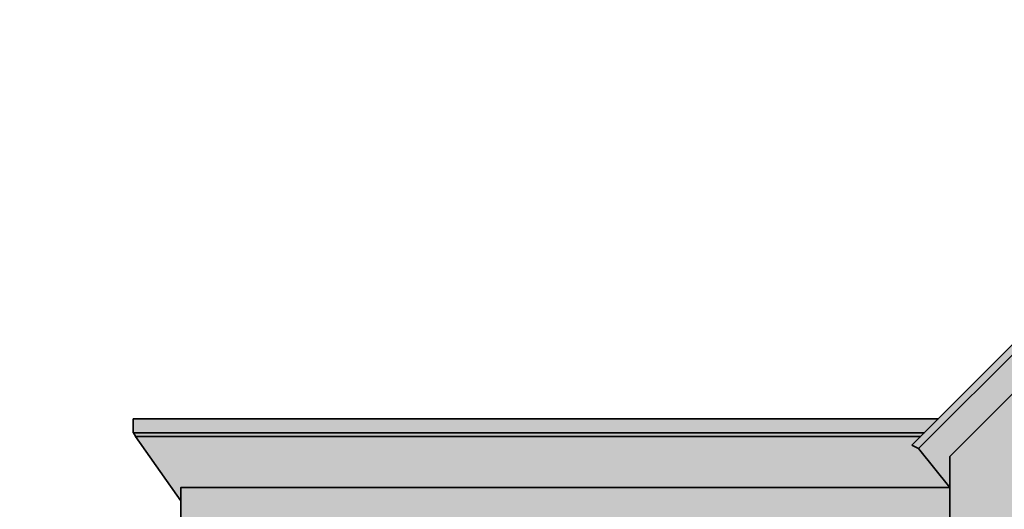
# Model space of a CAD drawing. Units: feet. Extents: x 2613 to 3913, y 950 to 1393.
# Tile 4 of 6: x 2613 to 2948, y 1226 to 1393. Entities that reach past the tile are written whole.
import ezdxf

# ---------------------------------------------------------------- set-up
doc = ezdxf.new("R2010")
doc.units = ezdxf.units.FT
for name, color, linetype, lineweight in [('A-ELEV', 7, 'Continuous', 35), ('A-ELEV-PATT', 9, 'Continuous', 13), ('A-ROOF', 1, 'Continuous', 35)]:
    doc.layers.add(name, color=color, linetype=linetype, lineweight=lineweight)

msp = doc.modelspace()

# ---------------------------------------------------------------- hatches: boundary and pattern name
at = {"layer": 'A-ELEV-PATT'}
h = msp.add_hatch(color=256, dxfattribs=at)
h.dxf.hatch_style = 1
h.paths.add_polyline_path([(3108.91, 1328.81), (3061.44, 1376.28), (2929.45, 1244.29), (2929.45, 1223.38), (2942.09, 1223.38), (2942.09, 1215.5), (2929.45, 1215.5), (2929.45, 1084.12), (3108.91, 1084.12), (3108.91, 1199.69), (3106.87, 1199.69), (3106.87, 1128.72), (3017.91, 1128.72), (3017.91, 1199.69), (3008.08, 1199.69), (3008.08, 1180.01), (3007.65, 1180.01), (3007.65, 1199.69), (3004.75, 1199.69), (3004.75, 1206.47), (3108.91, 1206.47)])
h.paths.add_polyline_path([(3061.44, 1376.28), (3193.8, 1243.92), (3193.8, 1233.84), (3204.34, 1246.9), (3061.54, 1389.71), (2918.82, 1247), (2929.45, 1233.69), (2929.45, 1244.29)])
h.paths.add_polyline_path([(3061.54, 1389.71), (3204.34, 1246.9), (3206.69, 1248.02), (3061.63, 1393.09), (2916.59, 1248.06), (2918.82, 1247)])
h.paths.add_polyline_path([(2925.65, 1257.12), (2667.59, 1257.12), (2651.33, 1257.12), (2651.33, 1252.28), (2920.82, 1252.28)])
h.paths.add_polyline_path([(2920.82, 1252.28), (2651.33, 1252.28, -0.144454), (2652.15, 1251.12), (2667.59, 1251.12), (2919.65, 1251.12)])
h.paths.add_polyline_path([(2918.82, 1247), (2916.59, 1248.06), (2919.65, 1251.12), (2667.59, 1251.12), (2652.15, 1251.12), (2667.59, 1229.14), (2667.59, 1233.69), (2929.45, 1233.69)])
h.paths.add_polyline_path([(2710.6, 1223.38), (2929.45, 1223.38), (2929.45, 1233.69), (2667.59, 1233.69), (2667.59, 1229.14), (2667.59, 1201.16), (2720.67, 1201.16), (2710.6, 1215.5)])
h.paths.add_polyline_path([(2942.09, 1223.38), (2710.6, 1223.38), (2710.6, 1215.5), (2921.48, 1215.5), (2942.09, 1215.5)])
h.paths.add_polyline_path([(2929.45, 1215.5), (2921.48, 1215.5), (2710.6, 1215.5), (2733.47, 1182.94), (2733.47, 1195.74), (2741.22, 1195.74), (2929.45, 1195.74)])
h.paths.add_polyline_path([(2721, 1200.68), (2661.89, 1200.68), (2661.89, 1195.74), (2724.47, 1195.74)])
h.paths.add_polyline_path([(2733.47, 1182.94), (2727.27, 1191.76), (2727.27, 1133.88), (2731.7, 1133.88), (2731.7, 1169.74), (2731.61, 1169.74), (2731.61, 1170.13), (2733.47, 1170.13)])
h.paths.add_polyline_path([(2929.45, 1183.04), (2741.22, 1183.04), (2741.22, 1170.13), (2743.07, 1170.13), (2743.07, 1169.74), (2743.07, 1112.32), (2759.57, 1112.32), (2759.57, 1167.82), (2763.7, 1167.82), (2763.7, 1112.32), (2781.75, 1112.32), (2781.75, 1167.82), (2785.87, 1167.82), (2785.87, 1112.32), (2803.92, 1112.32), (2803.92, 1167.82), (2808.05, 1167.82), (2808.05, 1112.32), (2826.09, 1112.32), (2826.09, 1167.82), (2830.22, 1167.82), (2830.22, 1112.32), (2875.17, 1112.32), (2875.17, 1171.49), (2929.45, 1171.49)])
h.paths.add_polyline_path([(2731.7, 1133.88), (2661.89, 1133.88), (2661.89, 1084.12), (2730.99, 1084.12), (2730.99, 1112.32), (2731.7, 1112.32)])
h.paths.add_polyline_path([(2929.45, 1112.32), (2730.99, 1112.32), (2730.99, 1084.12), (2929.45, 1084.12)])
h.paths.add_polyline_path([(2929.45, 1084.12), (2730.99, 1084.12), (2661.89, 1084.12), (2612.72, 1084.12), (2612.72, 1082.68), (2929.45, 1082.68)])
h.paths.add_polyline_path([(2929.45, 1082.68), (2612.72, 1082.68), (2639.32, 1062.44), (2733.47, 1062.44), (2733.47, 1063.35), (2639.62, 1063.35), (2615.43, 1081.77), (2723.91, 1081.77), (2739.71, 1069.74), (2741.22, 1069.74), (2725.42, 1081.77), (2929.45, 1081.77)])
h.paths.add_polyline_path([(2671.42, 1081.77), (2668.07, 1081.77), (2692.27, 1063.35), (2695.62, 1063.35)], flags=17)
h.paths.add_polyline_path([(2741.22, 1069.74), (2741.22, 1068.59), (2748.11, 1063.35), (2741.22, 1063.35), (2741.22, 1062.44), (2750.82, 1062.44)], flags=17)
h.paths.add_polyline_path([(2929.45, 1081.77), (2725.42, 1081.77), (2750.82, 1062.44), (2741.22, 1062.44), (2741.22, 1047.95), (2743.07, 1047.95), (2743.07, 1047.56), (2743.07, 967.97), (2875.17, 967.97), (2875.17, 1066.37), (2929.45, 1066.37)])
h.paths.add_polyline_path([(2778.55, 1066.37), (2806.94, 1066.37), (2806.94, 982.04), (2778.55, 982.04)], flags=16)
h.paths.add_polyline_path([(2778.55, 1064.05), (2806.94, 1064.05), (2806.94, 1063.39), (2778.55, 1063.39)], flags=16)
h.paths.add_polyline_path([(2778.55, 1061.07), (2806.94, 1061.07), (2806.94, 1060.41), (2778.55, 1060.41)], flags=0)
h.paths.add_polyline_path([(2778.55, 1058.09), (2806.94, 1058.09), (2806.94, 1057.43), (2778.55, 1057.43)], flags=0)
h.paths.add_polyline_path([(2778.55, 1055.11), (2806.94, 1055.11), (2806.94, 1054.45), (2778.55, 1054.45)], flags=0)
h.paths.add_polyline_path([(2778.55, 1052.13), (2806.94, 1052.13), (2806.94, 1051.47), (2778.55, 1051.47)], flags=0)
h.paths.add_polyline_path([(2778.55, 1049.15), (2806.94, 1049.15), (2806.94, 1048.49), (2778.55, 1048.49)], flags=0)
h.paths.add_polyline_path([(2778.55, 1046.18), (2806.94, 1046.18), (2806.94, 1045.51), (2778.55, 1045.51)], flags=0)
h.paths.add_polyline_path([(2778.55, 1043.2), (2806.94, 1043.2), (2806.94, 1042.53), (2778.55, 1042.53)], flags=0)
h.paths.add_polyline_path([(2778.55, 1040.22), (2806.94, 1040.22), (2806.94, 1039.56), (2778.55, 1039.56)], flags=0)
h.paths.add_polyline_path([(2778.55, 1037.24), (2806.94, 1037.24), (2806.94, 1036.58), (2778.55, 1036.58)], flags=0)
h.paths.add_polyline_path([(2778.55, 1034.26), (2806.94, 1034.26), (2806.94, 1033.6), (2778.55, 1033.6)], flags=0)
h.paths.add_polyline_path([(2778.55, 1031.28), (2806.94, 1031.28), (2806.94, 1030.62), (2778.55, 1030.62)], flags=0)
h.paths.add_polyline_path([(2778.55, 1028.3), (2806.94, 1028.3), (2806.94, 1027.64), (2778.55, 1027.64)], flags=0)
h.paths.add_polyline_path([(2778.55, 1025.32), (2806.94, 1025.32), (2806.94, 1024.66), (2778.55, 1024.66)], flags=0)
h.paths.add_polyline_path([(2778.55, 1022.34), (2806.94, 1022.34), (2806.94, 1021.68), (2778.55, 1021.68)], flags=0)
h.paths.add_polyline_path([(2778.55, 1019.36), (2806.94, 1019.36), (2806.94, 1018.7), (2778.55, 1018.7)], flags=0)
h.paths.add_polyline_path([(2778.55, 1016.71), (2806.94, 1016.71), (2806.94, 1016.05), (2778.55, 1016.05)], flags=0)
h.paths.add_polyline_path([(2824.02, 1066.37), (2852.41, 1066.37), (2852.41, 982.04), (2824.02, 982.04)], flags=16)
h.paths.add_polyline_path([(2778.55, 1014.07), (2806.94, 1014.07), (2806.94, 1013.4), (2778.55, 1013.4)], flags=0)
h.paths.add_polyline_path([(2824.02, 1064.05), (2852.41, 1064.05), (2852.41, 1063.39), (2824.02, 1063.39)], flags=16)
h.paths.add_polyline_path([(2824.02, 1061.07), (2852.41, 1061.07), (2852.41, 1060.41), (2824.02, 1060.41)], flags=0)
h.paths.add_polyline_path([(2824.02, 1058.09), (2852.41, 1058.09), (2852.41, 1057.43), (2824.02, 1057.43)], flags=0)
h.paths.add_polyline_path([(2824.02, 1055.11), (2852.41, 1055.11), (2852.41, 1054.45), (2824.02, 1054.45)], flags=16)
h.paths.add_polyline_path([(2824.02, 1052.13), (2852.41, 1052.13), (2852.41, 1051.47), (2824.02, 1051.47)], flags=0)
h.paths.add_polyline_path([(2778.55, 1011.09), (2806.94, 1011.09), (2806.94, 1010.43), (2778.55, 1010.43)], flags=0)
h.paths.add_polyline_path([(2824.02, 1049.15), (2852.41, 1049.15), (2852.41, 1048.49), (2824.02, 1048.49)], flags=0)
h.paths.add_polyline_path([(2824.02, 1046.18), (2852.41, 1046.18), (2852.41, 1045.51), (2824.02, 1045.51)], flags=0)
h.paths.add_polyline_path([(2824.02, 1043.2), (2852.41, 1043.2), (2852.41, 1042.53), (2824.02, 1042.53)], flags=0)
h.paths.add_polyline_path([(2778.55, 1008.11), (2806.94, 1008.11), (2806.94, 1007.45), (2778.55, 1007.45)], flags=0)
h.paths.add_polyline_path([(2824.02, 1040.22), (2852.41, 1040.22), (2852.41, 1039.56), (2824.02, 1039.56)], flags=0)
h.paths.add_polyline_path([(2824.02, 1037.24), (2852.41, 1037.24), (2852.41, 1036.58), (2824.02, 1036.58)], flags=0)
h.paths.add_polyline_path([(2778.55, 1005.13), (2806.94, 1005.13), (2806.94, 1004.47), (2778.55, 1004.47)], flags=0)
h.paths.add_polyline_path([(2824.02, 1034.26), (2852.41, 1034.26), (2852.41, 1033.6), (2824.02, 1033.6)], flags=0)
h.paths.add_polyline_path([(2824.02, 1031.28), (2852.41, 1031.28), (2852.41, 1030.62), (2824.02, 1030.62)], flags=0)
h.paths.add_polyline_path([(2778.55, 1002.15), (2806.94, 1002.15), (2806.94, 1001.49), (2778.55, 1001.49)], flags=0)
h.paths.add_polyline_path([(2824.02, 1028.3), (2852.41, 1028.3), (2852.41, 1027.64), (2824.02, 1027.64)], flags=0)
h.paths.add_polyline_path([(2778.55, 999.17), (2806.94, 999.17), (2806.94, 998.51), (2778.55, 998.51)], flags=0)
h.paths.add_polyline_path([(2824.02, 1025.32), (2852.41, 1025.32), (2852.41, 1024.66), (2824.02, 1024.66)], flags=0)
h.paths.add_polyline_path([(2824.02, 1022.34), (2852.41, 1022.34), (2852.41, 1021.68), (2824.02, 1021.68)], flags=0)
h.paths.add_polyline_path([(2778.55, 996.19), (2806.94, 996.19), (2806.94, 995.53), (2778.55, 995.53)], flags=0)
h.paths.add_polyline_path([(2824.02, 1019.36), (2852.41, 1019.36), (2852.41, 1018.7), (2824.02, 1018.7)], flags=0)
h.paths.add_polyline_path([(2778.55, 993.21), (2806.94, 993.21), (2806.94, 992.55), (2778.55, 992.55)], flags=0)
h.paths.add_polyline_path([(2824.02, 1016.38), (2852.41, 1016.38), (2852.41, 1015.72), (2824.02, 1015.72)], flags=0)
h.paths.add_polyline_path([(2824.02, 1013.4), (2852.41, 1013.4), (2852.41, 1012.74), (2824.02, 1012.74)], flags=0)
h.paths.add_polyline_path([(2778.55, 990.23), (2806.94, 990.23), (2806.94, 989.57), (2778.55, 989.57)], flags=0)
h.paths.add_polyline_path([(2824.02, 1010.43), (2852.41, 1010.43), (2852.41, 1009.76), (2824.02, 1009.76)], flags=0)
h.paths.add_polyline_path([(2778.55, 987.25), (2806.94, 987.25), (2806.94, 986.59), (2778.55, 986.59)], flags=0)
h.paths.add_polyline_path([(2824.02, 1007.45), (2852.41, 1007.45), (2852.41, 1006.78), (2824.02, 1006.78)], flags=0)
h.paths.add_polyline_path([(2778.55, 984.27), (2806.94, 984.27), (2806.94, 983.61), (2778.55, 983.61)], flags=0)
h.paths.add_polyline_path([(2824.02, 1004.47), (2852.41, 1004.47), (2852.41, 1003.81), (2824.02, 1003.81)], flags=0)
h.paths.add_polyline_path([(2824.02, 1001.49), (2852.41, 1001.49), (2852.41, 1000.83), (2824.02, 1000.83)], flags=0)
h.paths.add_polyline_path([(2824.02, 998.51), (2852.41, 998.51), (2852.41, 997.85), (2824.02, 997.85)], flags=0)
h.paths.add_polyline_path([(2824.02, 995.53), (2852.41, 995.53), (2852.41, 994.87), (2824.02, 994.87)], flags=0)
h.paths.add_polyline_path([(2824.02, 992.55), (2852.41, 992.55), (2852.41, 991.89), (2824.02, 991.89)], flags=0)
h.paths.add_polyline_path([(2824.02, 989.57), (2852.41, 989.57), (2852.41, 988.91), (2824.02, 988.91)], flags=0)
h.paths.add_polyline_path([(2824.02, 986.59), (2852.41, 986.59), (2852.41, 985.93), (2824.02, 985.93)], flags=0)
h.paths.add_polyline_path([(2824.02, 983.61), (2852.41, 983.61), (2852.41, 982.95), (2824.02, 982.95)], flags=0)
h.paths.add_polyline_path([(2731.7, 1047.56), (2731.61, 1047.56), (2731.61, 1047.95), (2733.47, 1047.95), (2733.47, 1062.44), (2727.27, 1062.44), (2727.27, 1000.58), (2667.59, 1000.58), (2667.59, 1062.44), (2664.87, 1062.44), (2664.87, 965.01), (2730.76, 964.93), (2730.76, 967.97), (2731.7, 967.97)])
h.paths.add_polyline_path([(2728.06, 961.9), (2730.76, 961.9), (2730.76, 964.93), (2663.94, 964.93), (2663.94, 949.74), (2725.36, 949.74), (2725.36, 955.82), (2728.06, 955.82)])
h.paths.add_polyline_path([(2929.45, 967.97), (2730.76, 967.97), (2730.76, 961.9), (2929.45, 961.9)])
h.paths.add_polyline_path([(2929.45, 961.9), (2730.76, 961.9), (2728.06, 961.9), (2728.06, 955.82), (2929.45, 955.82)])
h.paths.add_polyline_path([(2929.45, 955.82), (2728.06, 955.82), (2725.36, 955.82), (2725.36, 949.74), (2929.45, 949.74)])
h.paths.add_polyline_path([(2741.22, 1069.74), (2733.47, 1069.74), (2733.47, 1047.95), (2741.22, 1047.95)], flags=17)
h.paths.add_polyline_path([(2741.22, 1195.74), (2733.47, 1195.74), (2733.47, 1182.94), (2733.47, 1170.13), (2741.22, 1170.13), (2741.22, 1183.04)])
h.paths.add_polyline_path([(3193.8, 1084.12), (2929.45, 1084.12), (2929.45, 1082.68), (2929.45, 1081.77), (2929.45, 1066.37), (2929.45, 949.74), (3193.8, 949.74)])
h.paths.add_polyline_path([(2937.79, 1075.78), (3185.46, 1075.78), (3185.46, 958.09), (2937.79, 958.09)], flags=16)
h.paths.add_polyline_path([(3011.76, 1075.78), (3104.46, 1075.78), (3104.46, 993.6), (3011.76, 993.6)], flags=0)
h.paths.add_polyline_path([(3015.24, 1075.78), (3016.57, 1075.78), (3016.57, 1060.85), (3043.1, 1060.85), (3043.1, 1075.78), (3045.77, 1075.78), (3045.77, 997.08), (3070.45, 997.08), (3070.45, 1075.78), (3073.12, 1075.78), (3073.12, 1060.85), (3099.64, 1060.85), (3099.64, 1075.78), (3100.98, 1075.78), (3100.98, 997.08), (3099.64, 997.08), (3015.24, 997.08)], flags=0)

# ---------------------------------------------------------------- linework, layer by layer
at = {"layer": 'A-ELEV'}
for p, q in [((2667.59, 1229.14), (2652.15, 1251.12)), ((2667.59, 1229.14), (2652.15, 1251.12)), ((2929.45, 1233.69), (2918.82, 1247)), ((2929.45, 1233.69), (2918.82, 1247))]:
    msp.add_line(p, q, dxfattribs=at)
for points in [[(2929.45, 1244.29), (2929.45, 1223.38)], [(2929.45, 1244.29), (2929.45, 1223.38)], [(2929.45, 1233.69), (2667.59, 1233.69), (2667.59, 1229.14), (2667.59, 1201.16)], [(2929.45, 1233.69), (2667.59, 1233.69), (2667.59, 1229.14), (2667.59, 1201.16)]]:
    msp.add_lwpolyline(points, dxfattribs=at)
at = {"layer": 'A-ROOF'}
for p, q in [((3061.54, 1389.71), (2918.82, 1247)), ((3061.54, 1389.71), (2918.82, 1247)), ((2929.45, 1244.29), (3061.44, 1376.28)), ((2929.45, 1244.29), (3061.44, 1376.28)), ((2667.59, 1257.12), (2651.33, 1257.12)), ((2651.33, 1252.28), (2651.33, 1257.12)), ((2667.59, 1257.12), (2651.33, 1257.12)), ((2651.33, 1252.28), (2651.33, 1257.12)), ((2925.65, 1257.12), (2667.59, 1257.12)), ((2925.65, 1257.12), (2667.59, 1257.12)), ((2920.82, 1252.28), (2651.33, 1252.28)), ((2920.82, 1252.28), (2651.33, 1252.28)), ((2667.59, 1251.12), (2652.15, 1251.12)), ((2667.59, 1251.12), (2652.15, 1251.12)), ((2667.59, 1251.12), (2919.65, 1251.12)), ((2667.59, 1251.12), (2919.65, 1251.12)), ((2918.82, 1247), (2916.59, 1248.06)), ((2918.82, 1247), (2916.59, 1248.06))]:
    msp.add_line(p, q, dxfattribs=at)
msp.add_lwpolyline([(3206.69, 1248.02), (3061.63, 1393.09), (2916.59, 1248.06)], dxfattribs=at)
msp.add_lwpolyline([(3206.69, 1248.02), (3061.63, 1393.09), (2916.59, 1248.06)], dxfattribs=at)
msp.add_arc((2649.77, 1250.31), 2.52, 18.6443, 51.5233, dxfattribs=at)
msp.add_arc((2649.77, 1250.31), 2.52, 18.6443, 51.5233, dxfattribs=at)

doc.saveas('drawing.dxf')
